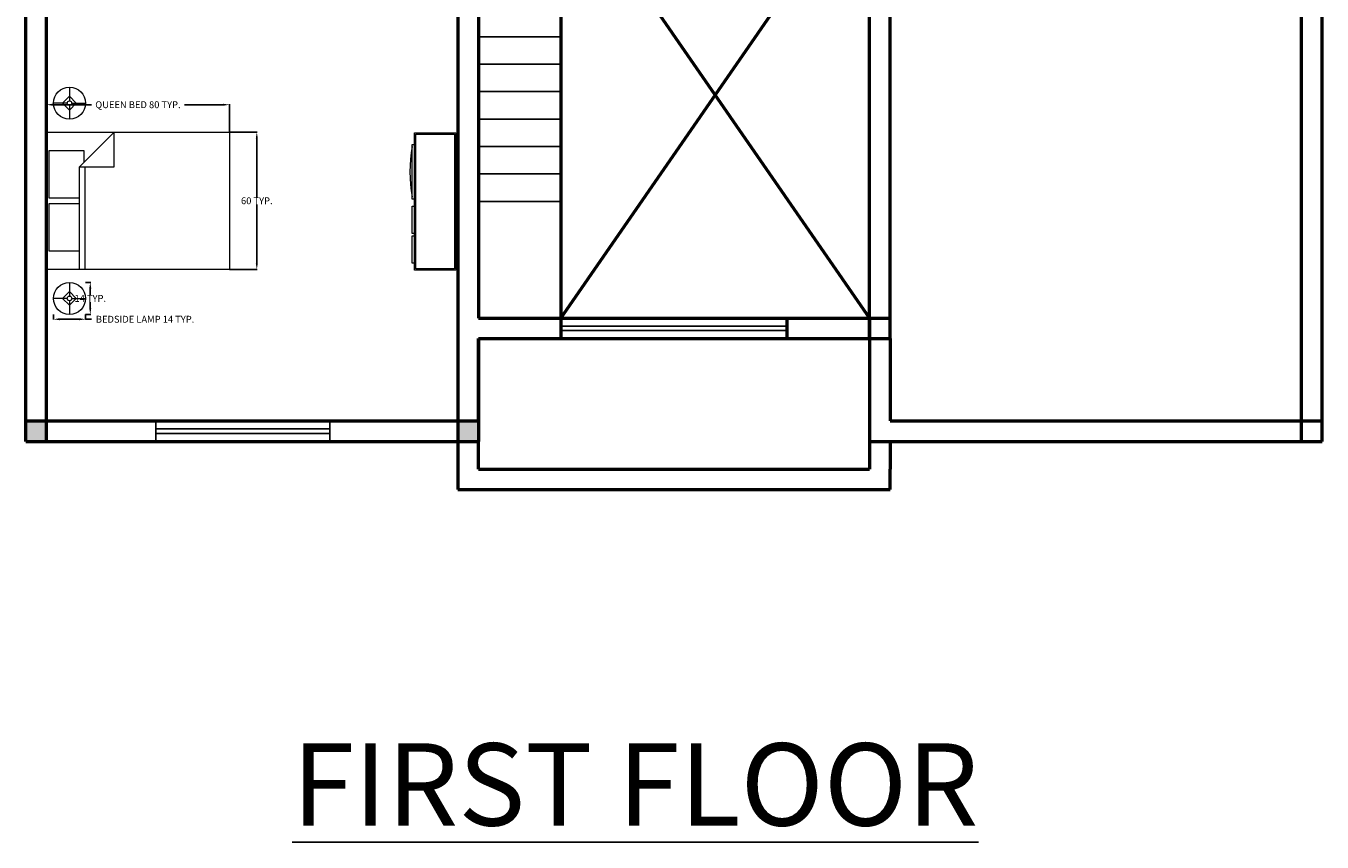
# Model space of a CAD drawing. Units: inches. Extents: x 13 to 1693, y -7 to 1519.
# Tile 8 of 10: x 1126 to 1693, y -7 to 350. Entities that reach past the tile are written whole.
import ezdxf

# ---------------------------------------------------------------- set-up
doc = ezdxf.new("R2010")
doc.units = ezdxf.units.IN
doc.header["$MEASUREMENT"] = 0
for name, color, linetype, lineweight in [('A-ANNO-DIMS', 2, 'Continuous', 18), ('A-ANNO-TEXT', 7, 'Continuous', 25), ('A-FLOR-STRS', 2, 'Continuous', 25), ('A-FURN', 8, 'Continuous', 18), ('A-GLAZ', 4, 'Continuous', 25), ('A-WALL', 7, 'Continuous', 50), ('A-WALL-PATT', 8, 'Continuous', 13)]:
    doc.layers.add(name, color=color, linetype=linetype, lineweight=lineweight)
doc.styles.get("Standard").update_dxf_attribs({"font": 'arial.ttf'})
doc.dimstyles.get("Standard").update_dxf_attribs({"dimtxt": 3, "dimasz": 2.68, "dimexe": 0.18, "dimexo": 0.0625, "dimgap": 0.09, "dimtad": 0, "dimtih": 1, "dimtoh": 1, "dimdec": 0, "dimzin": 0, "dimdsep": 46, "dimlunit": 3, "dimtxsty": 'Standard', "dimcen": 0.09, "dimadec": 0, "dimazin": 0, "dimtfac": 1, "dimtdec": 0, "dimtofl": 0, "dimtmove": 0, "dimatfit": 3, "dimfxl": 1, "dimtolj": 1, "dimtzin": 0, "dimarcsym": 0})

# ---------------------------------------------------------------- blocks, each defined once
blk = doc.blocks.new('Bed - Queen')
for p, q in [((0, -80.00003), (0, 0)), ((0, 0), (59.99999, 0)), ((59.99999, 0), (59.99999, -80.00003)), ((7.99999, -1.2), (28.79998, -1.2)), ((7.99999, -14.4), (7.99999, -1.2)), ((28.79998, -1.2), (28.79998, -14.4)), ((31.19999, -1.2), (51.99999, -1.2)), ((31.19999, -14.4), (31.19999, -1.2)), ((51.99999, -1.2), (51.99999, -16.4)), ((0, -14.4), (44.8, -14.4)), ((44.8, -16.8), (0, -16.8)), ((59.99999, -29.6), (44.8, -14.4)), ((44.8, -14.4), (44.8, -29.6)), ((51.99999, -16.4), (46.79936, -16.4)), ((44.8, -29.6), (59.99999, -29.6)), ((59.99999, -80.00003), (0, -80.00003))]:
    blk.add_line(p, q)
blk = doc.blocks.new('Lamp - Table')
for p, q in [((0, 7), (0, 1)), ((-1, 0), (-7, 0)), ((0, 3), (-3, 0)), ((-3, 0), (0, -3)), ((3, 0), (0, 3)), ((0, -3), (3, 0)), ((1, 0), (7, 0)), ((0, -1), (0, -7))]:
    blk.add_line(p, q)
for radius in [7, 1]:
    blk.add_circle((0, 0), radius)
blk = doc.blocks.new('Entertainment Center')
for p, q in [((-4, 0), (-5, -1)), ((4, 0), (-4, 0)), ((5, -1), (4, 0)), ((-17, -19), (-17, -1)), ((-17, -1), (43, -1)), ((-16.5, -18.5), (-16.5, -1.5)), ((-16.5, -1.5), (42.5, -1.5)), ((42.5, -1.5), (42.5, -18.5)), ((43, -1), (43, -19)), ((43, -19), (-17, -19)), ((42.5, -18.5), (-16.5, -18.5)), ((-12, -20), (-12, -19)), ((12, -20), (-12, -20)), ((12, -19), (12, -20)), ((15, -20), (15, -19)), ((27, -20), (15, -20)), ((27, -19), (27, -20)), ((28, -20), (28, -19)), ((40, -20), (28, -20)), ((40, -19), (40, -20))]:
    blk.add_line(p, q)
blk.add_arc((0, 40), 61, 259.6111, 280.3889)
blk = doc.blocks.new('WIN-76')
for p, q in [((0, 9), (0, 0)), ((76.02, 9), (76.02, 0)), ((0, 5.5), (76.02, 5.5)), ((0, 3.5), (76.02, 3.5))]:
    blk.add_line(p, q)
blk = doc.blocks.new('*D38')
at = {"layer": 'A-ANNO-DIMS', "color": 0, "lineweight": -2, "transparency": 16777216}
for p, q in [((1135.28, 303.51), (1135.28, 315.62)), ((1137.96, 315.44), (1154.97, 315.44)), ((1212.6, 315.44), (1195.59, 315.44)), ((1215.28, 303.51), (1215.28, 315.62))]:
    blk.add_line(p, q, dxfattribs=at)
at = {"layer": 'A-ANNO-DIMS', "color": 0, "transparency": 16777216}
for points in [[(1137.96, 315.89), (1137.96, 315), (1135.28, 315.44)], [(1212.6, 315.89), (1212.6, 315), (1215.28, 315.44)]]:
    blk.add_solid(points, dxfattribs=at)
at = {"layer": 'Defpoints', "color": 0, "transparency": 16777216}
for p in [(1135.28, 315.44), (1135.28, 303.44), (1215.28, 303.44)]:
    blk.add_point(p, dxfattribs=at)
at = {"layer": 'A-ANNO-DIMS', "color": 0, "transparency": 16777216, "insert": (1175.28, 315.44), "char_height": 3, "attachment_point": 5}
blk.add_mtext('\\A1;QUEEN BED 80 TYP.', dxfattribs=at)
blk = doc.blocks.new('*D39')
at = {"layer": 'A-ANNO-DIMS', "color": 0, "lineweight": -2, "transparency": 16777216}
for p, q in [((1215.34, 303.44), (1227.46, 303.44)), ((1227.28, 300.76), (1227.28, 275.07)), ((1227.28, 246.12), (1227.28, 271.82)), ((1215.34, 243.44), (1227.46, 243.44))]:
    blk.add_line(p, q, dxfattribs=at)
at = {"layer": 'A-ANNO-DIMS', "color": 0, "transparency": 16777216}
for points in [[(1226.83, 300.76), (1227.73, 300.76), (1227.28, 303.44)], [(1226.83, 246.12), (1227.73, 246.12), (1227.28, 243.44)]]:
    blk.add_solid(points, dxfattribs=at)
at = {"layer": 'Defpoints', "color": 0, "transparency": 16777216}
for p in [(1215.28, 303.44), (1227.28, 303.44), (1215.28, 243.44)]:
    blk.add_point(p, dxfattribs=at)
at = {"layer": 'A-ANNO-DIMS', "color": 0, "transparency": 16777216, "insert": (1227.28, 273.44), "char_height": 3, "attachment_point": 5}
blk.add_mtext('\\A1;60 TYP.', dxfattribs=at)
blk = doc.blocks.new('*D42')
at = {"layer": 'A-ANNO-DIMS', "color": 0, "lineweight": -2, "transparency": 16777216}
for p, q in [((1138.33, 223.68), (1138.33, 221.46)), ((1141.01, 221.64), (1149.65, 221.64)), ((1152.33, 223.68), (1152.33, 221.46)), ((1152.33, 221.64), (1155.01, 221.64))]:
    blk.add_line(p, q, dxfattribs=at)
at = {"layer": 'A-ANNO-DIMS', "color": 0, "transparency": 16777216}
for points in [[(1141.01, 222.09), (1141.01, 221.19), (1138.33, 221.64)], [(1149.65, 222.09), (1149.65, 221.19), (1152.33, 221.64)]]:
    blk.add_solid(points, dxfattribs=at)
at = {"layer": 'Defpoints', "color": 0, "transparency": 16777216}
for p in [(1138.33, 223.74), (1152.33, 223.74), (1152.33, 221.64)]:
    blk.add_point(p, dxfattribs=at)
at = {"layer": 'A-ANNO-DIMS', "color": 0, "transparency": 16777216, "insert": (1178.41, 221.64), "char_height": 3, "attachment_point": 5}
blk.add_mtext('\\A1;BEDSIDE LAMP 14 TYP.', dxfattribs=at)
blk = doc.blocks.new('*D43')
at = {"layer": 'A-ANNO-DIMS', "color": 0, "lineweight": -2, "transparency": 16777216}
for p, q in [((1152.39, 237.74), (1154.61, 237.74)), ((1154.43, 235.06), (1154.43, 232.34)), ((1154.43, 226.42), (1154.43, 229.14)), ((1152.39, 223.74), (1154.61, 223.74))]:
    blk.add_line(p, q, dxfattribs=at)
at = {"layer": 'A-ANNO-DIMS', "color": 0, "transparency": 16777216}
for points in [[(1153.98, 235.06), (1154.88, 235.06), (1154.43, 237.74)], [(1153.98, 226.42), (1154.88, 226.42), (1154.43, 223.74)]]:
    blk.add_solid(points, dxfattribs=at)
at = {"layer": 'Defpoints', "color": 0, "transparency": 16777216}
for p in [(1152.33, 237.74), (1154.43, 237.74), (1152.33, 223.74)]:
    blk.add_point(p, dxfattribs=at)
at = {"layer": 'A-ANNO-DIMS', "color": 0, "transparency": 16777216, "insert": (1154.43, 230.74), "char_height": 3, "attachment_point": 5}
blk.add_mtext('\\A1;14 TYP.', dxfattribs=at)

msp = doc.modelspace()

# ---------------------------------------------------------------- hatches: boundary and pattern name
at = {"layer": 'A-WALL-PATT'}
h = msp.add_hatch(color=256, dxfattribs=at)
h.dxf.hatch_style = 1
h.paths.add_polyline_path([(1135.28, 735.15), (1126.28, 735.15), (1126.28, 726.15), (1135.28, 726.15)])
h.paths.add_polyline_path([(1135.28, 657.15), (1126.28, 657.15), (1126.28, 648.15), (1135.28, 648.15)])
h.paths.add_polyline_path([(1135.28, 498.15), (1126.28, 498.15), (1126.28, 489.15), (1135.28, 489.15)])
h.paths.add_polyline_path([(1135.28, 417.15), (1126.28, 417.15), (1126.28, 408.15), (1135.28, 408.15)])
h.paths.add_polyline_path([(1135.28, 177.15), (1126.28, 177.15), (1126.28, 168.15), (1135.28, 168.15)])
h.paths.add_polyline_path([(1324.28, 177.15), (1315.28, 177.15), (1315.28, 168.15), (1324.28, 168.15)])
h.paths.add_polyline_path([(1324.28, 417.15), (1315.28, 417.15), (1315.28, 408.15), (1324.28, 408.15)])
h.paths.add_polyline_path([(1324.28, 498.15), (1315.28, 498.15), (1315.28, 489.15), (1324.28, 489.15)])
h.paths.add_polyline_path([(1324.28, 657.15), (1315.28, 657.15), (1315.28, 648.15), (1324.28, 648.15)])

# ---------------------------------------------------------------- linework, layer by layer
at = {"layer": 'A-FLOR-STRS'}
for p, q in [((1324.28, 345.15), (1360.28, 345.15)), ((1324.28, 333.15), (1360.28, 333.15)), ((1324.28, 321.15), (1360.28, 321.15)), ((1324.28, 309.15), (1360.28, 309.15)), ((1324.28, 297.15), (1360.28, 297.15)), ((1324.28, 285.15), (1360.28, 285.15)), ((1324.28, 273.15), (1360.28, 273.15))]:
    msp.add_line(p, q, dxfattribs=at)
at = {"layer": 'A-GLAZ'}
for p, q in [((1360.28, 218.65), (1459.28, 218.65)), ((1360.28, 216.65), (1459.28, 216.65))]:
    msp.add_line(p, q, dxfattribs=at)
at = {"layer": 'A-WALL'}
for p, q in [((1126.28, 168.15), (1126.28, 735.15)), ((1693.28, 168.15), (1693.28, 735.15)), ((1315.28, 417.15), (1315.28, 168.15)), ((1324.28, 417.15), (1324.28, 222.15)), ((1360.28, 417.15), (1360.28, 222.15)), ((1360.28, 417.15), (1495.28, 222.15)), ((1360.28, 222.15), (1495.28, 417.15)), ((1495.28, 213.15), (1495.28, 417.15)), ((1504.28, 213.15), (1504.28, 408.15)), ((1135.28, 168.15), (1135.28, 360.15)), ((1684.28, 168.15), (1684.28, 360.15)), ((1324.28, 222.15), (1459.28, 222.15)), ((1360.28, 222.15), (1360.28, 213.15)), ((1459.28, 222.15), (1504.28, 222.15)), ((1459.28, 213.15), (1459.28, 222.15)), ((1495.28, 222.15), (1495.28, 156.15)), ((1324.28, 213.15), (1324.28, 168.15)), ((1324.28, 177.15), (1324.28, 213.15)), ((1324.28, 213.15), (1504.28, 213.15)), ((1504.28, 213.15), (1504.28, 177.15)), ((1126.28, 177.15), (1324.28, 177.15)), ((1504.28, 177.15), (1693.28, 177.15)), ((1126.28, 168.15), (1324.28, 168.15)), ((1315.28, 168.15), (1315.28, 156.15)), ((1324.28, 156.15), (1324.28, 168.15)), ((1495.28, 168.15), (1693.28, 168.15)), ((1504.28, 168.15), (1504.28, 156.15)), ((1315.28, 156.15), (1315.28, 147.15)), ((1324.28, 156.15), (1495.28, 156.15)), ((1504.28, 147.15), (1504.28, 156.15)), ((1315.28, 147.15), (1324.28, 147.15)), ((1324.28, 147.15), (1504.28, 147.15))]:
    msp.add_line(p, q, dxfattribs=at)
msp.add_lwpolyline([(1360.28, 222.15), (1495.28, 222.15), (1495.28, 417.15), (1360.28, 417.15)], close=True, dxfattribs=at)

# ---------------------------------------------------------------- block references
at = {"layer": 'A-FURN'}
for p in [(1145.33, 316.12), (1145.33, 230.74)]:
    msp.add_blockref('Lamp - Table', p, dxfattribs=at)
for name, p, rotation in [('Bed - Queen', (1135.28, 243.44), 90), ('Entertainment Center', (1315.28, 286.11), 270)]:
    msp.add_blockref(name, p, dxfattribs=dict(at, rotation=rotation))
at = {"layer": 'A-GLAZ'}
msp.add_blockref('WIN-76', (1183.17, 168.15), dxfattribs=at)

# ---------------------------------------------------------------- texts
at = {"layer": 'A-ANNO-TEXT', "insert": (1242.73, 36.23), "char_height": 36, "attachment_point": 1}
msp.add_mtext_dynamic_manual_height_columns('{\\LFIRST FLOOR}', width=444.8977, gutter_width=1, heights=[0], dxfattribs=at)

# ---------------------------------------------------------------- dimensions: what is measured, and where the dimension line sits
at = {"layer": 'A-ANNO-DIMS'}
for base, p1, p2, angle, text, picture, middle in [((1135.28, 315.44), (1215.28, 303.44), (1135.28, 303.44), 180, 'QUEEN BED <> TYP.', '*D38', (1175.28, 315.44)), ((1227.28, 303.44), (1215.28, 243.44), (1215.28, 303.44), 90, '<> TYP.', '*D39', (1227.28, 273.44)), ((1154.43, 237.74), (1152.33, 223.74), (1152.33, 237.74), 90, '<> TYP.', '*D43', (1154.43, 230.74))]:
    dim = msp.add_linear_dim(base=base, p1=p1, p2=p2, angle=angle, text=text, dimstyle='Standard', override={"dimdec": 0, "dimlfac": 1, "dimrnd": 0, "dimzin": 0, "dimdsep": 46, "dimlunit": 2}, dxfattribs=at)
    dim.commit()
    dim.dimension.update_dxf_attribs({"geometry": picture, "text_midpoint": middle})
dim = msp.add_linear_dim(base=(1152.33, 221.64), p1=(1138.33, 223.74), p2=(1152.33, 223.74), text='BEDSIDE LAMP <> TYP.', dimstyle='Standard', override={"dimdec": 0, "dimlfac": 1, "dimrnd": 0, "dimzin": 0, "dimdsep": 46, "dimlunit": 2}, dxfattribs=at)
dim.commit()
dim.dimension.update_dxf_attribs({"geometry": '*D42', "text_midpoint": (1178.41, 221.64)})

doc.saveas('drawing.dxf')
